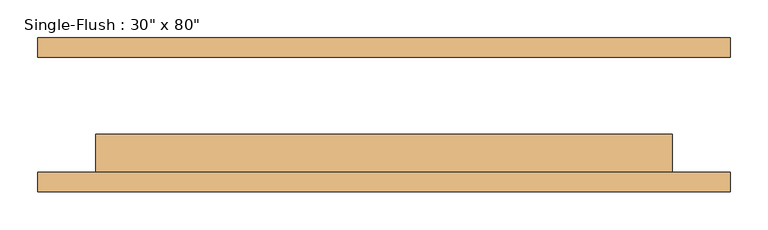
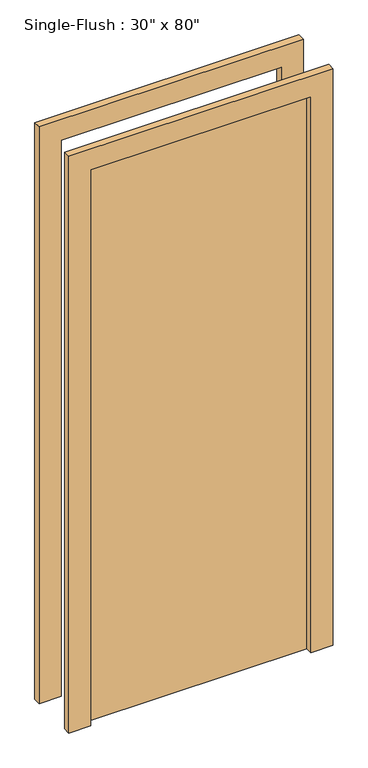
"""IFC4 building model written with IfcOpenShell, lengths in millimetres: door geometry."""

from ifc_helpers import new_model, si_unit, frame, origin, origin_with_axes, place, context, project, spatial, polyline, outline, extrude, source, transform, mapped, element, save


def door_255cab33(model_context):
    return source(origin(), model_context, "Body", "SweptSolid", [
        extrude(outline(polyline([(2108.2, -457.2), (0.0, -457.2), (0.0, -381.0), (2032.0, -381.0), (2032.0, 381.0), (0.0, 381.0), (0.0, 457.2), (2108.2, 457.2), (2108.2, -457.2)])), frame((0.0, -101.6, 0.0), z_axis=(0.0, 1.0, 0.0), x_axis=(0.0, 0.0, 1.0)), (0.0, 0.0, 1.0), 25.4),
        extrude(outline(polyline([(2108.2, 457.2), (2108.2, -457.2), (0.0, -457.2), (0.0, -381.0), (2032.0, -381.0), (2032.0, 381.0), (0.0, 381.0), (0.0, 457.2), (2108.2, 457.2)])), frame((0.0, 76.2, 0.0), z_axis=(0.0, 1.0, 0.0), x_axis=(0.0, 0.0, 1.0)), (0.0, 0.0, 1.0), 25.4),
        extrude(outline(polyline([(381.0, -25.4), (381.0, -76.2), (-381.0, -76.2), (-381.0, -25.4), (381.0, -25.4)])), origin_with_axes(), (0.0, 0.0, 1.0), 2032.0),
    ])


if __name__ == "__main__":
    model = new_model("IFC4")
    model_context = context("Model", 3, world=origin())
    ifc_project = project(units=[si_unit("LENGTHUNIT", "METRE", prefix="MILLI")], contexts=[model_context])
    site = spatial("IfcSite", under=ifc_project)
    building = spatial("IfcBuilding", under=site)
    placement = place(None, origin())
    door_shape = door_255cab33(model_context)
    element("IfcDoor", 1, ObjectType="Single-Flush : 30\" x 80\"", at=placement, inside=building, context=model_context, shape_type="MappedRepresentation", body=[
        mapped(door_shape, transform((0.0, 0.0, 0.0), x_axis=(1.0, 0.0, 0.0), y_axis=(0.0, 1.0, 0.0), z_axis=(0.0, 0.0, 1.0))),
    ])
    save(model, "model.ifc")

# Revit data of these elements
# Type "Single-Flush : 30\" x 80\""
#   Type Mark = "5"
#   Construction Type Id = "MDOOR"
#   Assembly Code = "C1020"
#   Analytic Construction = "Metal"
#   Thickness = 0' - 2"
#   Heat Transfer Coefficient (U) = 0.651978 BTU/(h·ft²·°F)
#   Height = 6' - 8"
#   Trim Projection Ext = 0' - 1"
#   Trim Projection Int = 0' - 1"
#   Trim Width = 0' - 3"
#   Width = 2' - 6"
#   Define Thermal Properties by = 1
#   Define Thermal Properties by = 1
#   Door Material = Door - Panel
#   Frame Material = Door - Frame
#   Visual Light Transmittance = 0
#   Solar Heat Gain Coefficient = 0
#   Function = (empty or 0)
#   Wall Closure = (empty or 0)
# Element 1 (IfcDoor, "Single-Flush : 30\" x 80\"")
#   Materials on its faces: "Door - Frame", "Door - Panel"
# Materials
#   "Door - Panel": class "Wood", colour RGB 210 159 95, transparency 0, Cost = 0
#   "Door - Frame": colour RGB 118 70 51, transparency 0, Cost = 0
